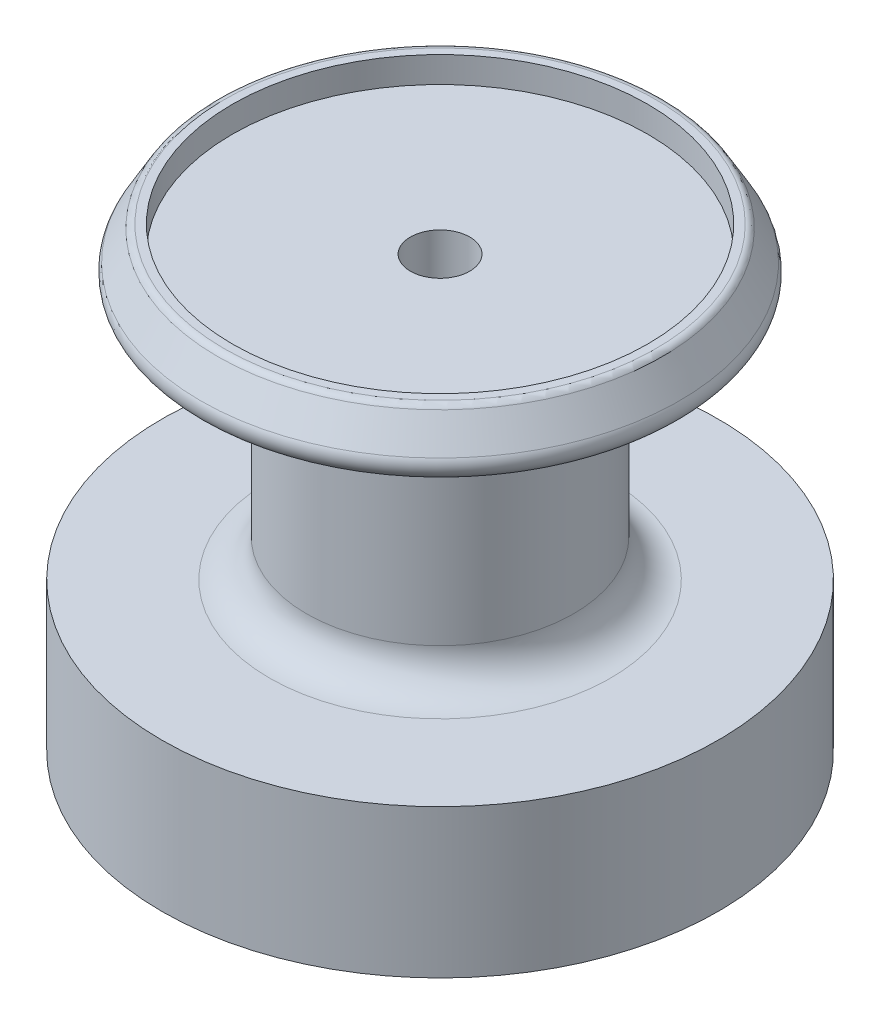
ISO-10303-21;
HEADER;
FILE_DESCRIPTION(('STEP AP214'),'2;1');
FILE_NAME('part.step','',(''),(''),'','','');
FILE_SCHEMA(('AUTOMOTIVE_DESIGN { 1 0 10303 214 1 1 1 1 }'));
ENDSEC;
DATA;
#1=APPLICATION_CONTEXT('core data for automotive mechanical design processes');
#2=APPLICATION_PROTOCOL_DEFINITION('international standard','automotive_design',2000,#1);
#3=PRODUCT_CONTEXT('',#1,'mechanical');
#4=PRODUCT('Part','Part','',(#3));
#5=PRODUCT_RELATED_PRODUCT_CATEGORY('part','',(#4));
#6=PRODUCT_DEFINITION_FORMATION('','',#4);
#7=PRODUCT_DEFINITION_CONTEXT('part definition',#1,'design');
#8=PRODUCT_DEFINITION('design','',#6,#7);
#9=PRODUCT_DEFINITION_SHAPE('','',#8);
#10=(LENGTH_UNIT() NAMED_UNIT(*) SI_UNIT(.MILLI.,.METRE.));
#11=(NAMED_UNIT(*) PLANE_ANGLE_UNIT() SI_UNIT($,.RADIAN.));
#12=(NAMED_UNIT(*) SI_UNIT($,.STERADIAN.) SOLID_ANGLE_UNIT());
#13=UNCERTAINTY_MEASURE_WITH_UNIT(LENGTH_MEASURE(1.E-05),#10,'distance_accuracy_value','');
#14=(GEOMETRIC_REPRESENTATION_CONTEXT(3) GLOBAL_UNCERTAINTY_ASSIGNED_CONTEXT((#13)) GLOBAL_UNIT_ASSIGNED_CONTEXT((#10,
#11,#12)) REPRESENTATION_CONTEXT('',''));
#15=CARTESIAN_POINT('',(0.,0.,0.));
#16=DIRECTION('',(0.,0.,1.));
#17=DIRECTION('',(1.,0.,0.));
#18=AXIS2_PLACEMENT_3D('',#15,#16,#17);
#19=CARTESIAN_POINT('',(0.,20.,0.));
#20=DIRECTION('',(0.,-1.,0.));
#21=DIRECTION('',(0.,0.,-1.));
#22=AXIS2_PLACEMENT_3D('',#19,#20,#21);
#23=CYLINDRICAL_SURFACE('',#22,37.5);
#24=CARTESIAN_POINT('',(0.,20.,0.));
#25=DIRECTION('',(0.,1.,0.));
#26=DIRECTION('',(0.,0.,1.));
#27=AXIS2_PLACEMENT_3D('',#24,#25,#26);
#28=CIRCLE('',#27,37.5);
#29=CARTESIAN_POINT('',(0.,20.,37.5));
#30=VERTEX_POINT('',#29);
#31=EDGE_CURVE('E62',#30,#30,#28,.T.);
#32=ORIENTED_EDGE('',*,*,#31,.F.);
#33=EDGE_LOOP('',(#32));
#34=FACE_BOUND('',#33,.T.);
#35=CARTESIAN_POINT('',(0.,0.,0.));
#36=DIRECTION('',(0.,1.,0.));
#37=DIRECTION('',(0.,0.,1.));
#38=AXIS2_PLACEMENT_3D('',#35,#36,#37);
#39=CIRCLE('',#38,37.5);
#40=CARTESIAN_POINT('',(0.,0.,37.5));
#41=VERTEX_POINT('',#40);
#42=EDGE_CURVE('E65',#41,#41,#39,.T.);
#43=ORIENTED_EDGE('',*,*,#42,.T.);
#44=EDGE_LOOP('',(#43));
#45=FACE_BOUND('',#44,.T.);
#46=ADVANCED_FACE('F40',(#34,#45),#23,.T.);
#47=CARTESIAN_POINT('',(0.,20.,0.));
#48=DIRECTION('',(0.,1.,0.));
#49=DIRECTION('',(0.,0.,1.));
#50=AXIS2_PLACEMENT_3D('',#47,#48,#49);
#51=PLANE('',#50);
#52=CARTESIAN_POINT('',(0.,20.,0.));
#53=DIRECTION('',(0.,1.,0.));
#54=DIRECTION('',(0.,0.,1.));
#55=AXIS2_PLACEMENT_3D('',#52,#53,#54);
#56=CIRCLE('',#55,23.);
#57=CARTESIAN_POINT('',(0.,20.,23.));
#58=VERTEX_POINT('',#57);
#59=EDGE_CURVE('E60',#58,#58,#56,.F.);
#60=ORIENTED_EDGE('',*,*,#59,.T.);
#61=EDGE_LOOP('',(#60));
#62=FACE_BOUND('',#61,.T.);
#63=ORIENTED_EDGE('',*,*,#31,.T.);
#64=EDGE_LOOP('',(#63));
#65=FACE_BOUND('',#64,.T.);
#66=ADVANCED_FACE('F148',(#62,#65),#51,.T.);
#67=CARTESIAN_POINT('',(0.,0.,0.));
#68=DIRECTION('',(0.,1.,0.));
#69=DIRECTION('',(0.,0.,1.));
#70=AXIS2_PLACEMENT_3D('',#67,#68,#69);
#71=PLANE('',#70);
#72=CARTESIAN_POINT('',(0.,0.,0.));
#73=DIRECTION('',(0.,-1.,0.));
#74=DIRECTION('',(0.,0.,-1.));
#75=AXIS2_PLACEMENT_3D('',#72,#73,#74);
#76=CIRCLE('',#75,35.);
#77=CARTESIAN_POINT('',(0.,0.,-35.));
#78=VERTEX_POINT('',#77);
#79=EDGE_CURVE('E79',#78,#78,#76,.T.);
#80=ORIENTED_EDGE('',*,*,#79,.F.);
#81=EDGE_LOOP('',(#80));
#82=FACE_BOUND('',#81,.T.);
#83=ORIENTED_EDGE('',*,*,#42,.F.);
#84=EDGE_LOOP('',(#83));
#85=FACE_BOUND('',#84,.T.);
#86=ADVANCED_FACE('F151',(#82,#85),#71,.F.);
#87=CARTESIAN_POINT('',(0.,54.,0.));
#88=DIRECTION('',(0.,-1.,0.));
#89=DIRECTION('',(0.,0.,-1.));
#90=AXIS2_PLACEMENT_3D('',#87,#88,#89);
#91=CYLINDRICAL_SURFACE('',#90,18.);
#92=CARTESIAN_POINT('',(0.,25.,0.));
#93=DIRECTION('',(0.,1.,0.));
#94=DIRECTION('',(0.,0.,1.));
#95=AXIS2_PLACEMENT_3D('',#92,#93,#94);
#96=CIRCLE('',#95,18.);
#97=CARTESIAN_POINT('',(0.,25.,18.));
#98=VERTEX_POINT('',#97);
#99=EDGE_CURVE('E58',#98,#98,#96,.T.);
#100=ORIENTED_EDGE('',*,*,#99,.T.);
#101=EDGE_LOOP('',(#100));
#102=FACE_BOUND('',#101,.T.);
#103=CARTESIAN_POINT('',(0.,54.,0.));
#104=DIRECTION('',(0.,1.,0.));
#105=DIRECTION('',(0.,0.,1.));
#106=AXIS2_PLACEMENT_3D('',#103,#104,#105);
#107=CIRCLE('',#106,18.);
#108=CARTESIAN_POINT('',(0.,54.,18.));
#109=VERTEX_POINT('',#108);
#110=EDGE_CURVE('E66',#109,#109,#107,.T.);
#111=ORIENTED_EDGE('',*,*,#110,.F.);
#112=EDGE_LOOP('',(#111));
#113=FACE_BOUND('',#112,.T.);
#114=ADVANCED_FACE('F158',(#102,#113),#91,.T.);
#115=CARTESIAN_POINT('',(0.,25.,0.));
#116=DIRECTION('',(0.,1.,0.));
#117=DIRECTION('',(0.,0.,1.));
#118=AXIS2_PLACEMENT_3D('',#115,#116,#117);
#119=TOROIDAL_SURFACE('',#118,23.,5.);
#120=ORIENTED_EDGE('',*,*,#59,.F.);
#121=EDGE_LOOP('',(#120));
#122=FACE_BOUND('',#121,.T.);
#123=ORIENTED_EDGE('',*,*,#99,.F.);
#124=EDGE_LOOP('',(#123));
#125=FACE_BOUND('',#124,.T.);
#126=ADVANCED_FACE('F141',(#122,#125),#119,.F.);
#127=CARTESIAN_POINT('',(0.,54.,0.));
#128=DIRECTION('',(0.,-1.,0.));
#129=DIRECTION('',(0.,0.,1.));
#130=AXIS2_PLACEMENT_3D('',#127,#128,#129);
#131=CONICAL_SURFACE('',#130,34.,0.523598775598299);
#132=CARTESIAN_POINT('',(0.,57.,0.));
#133=DIRECTION('',(0.,1.,0.));
#134=DIRECTION('',(0.,0.,1.));
#135=AXIS2_PLACEMENT_3D('',#132,#133,#134);
#136=CIRCLE('',#135,32.2679491924311);
#137=CARTESIAN_POINT('',(0.,57.,32.2679491924311));
#138=VERTEX_POINT('',#137);
#139=EDGE_CURVE('E42',#138,#138,#136,.T.);
#140=ORIENTED_EDGE('',*,*,#139,.T.);
#141=EDGE_LOOP('',(#140));
#142=FACE_BOUND('',#141,.T.);
#143=CARTESIAN_POINT('',(0.,61.,0.));
#144=DIRECTION('',(0.,-1.,0.));
#145=DIRECTION('',(0.,0.,-1.));
#146=AXIS2_PLACEMENT_3D('',#143,#144,#145);
#147=CIRCLE('',#146,29.9585481156726);
#148=CARTESIAN_POINT('',(0.,61.,-29.9585481156726));
#149=VERTEX_POINT('',#148);
#150=EDGE_CURVE('E48',#149,#149,#147,.T.);
#151=ORIENTED_EDGE('',*,*,#150,.T.);
#152=EDGE_LOOP('',(#151));
#153=FACE_BOUND('',#152,.T.);
#154=ADVANCED_FACE('F133',(#142,#153),#131,.T.);
#155=CARTESIAN_POINT('',(0.,61.5,0.));
#156=DIRECTION('',(0.,1.,0.));
#157=DIRECTION('',(0.,0.,1.));
#158=AXIS2_PLACEMENT_3D('',#155,#156,#157);
#159=PLANE('',#158);
#160=CARTESIAN_POINT('',(0.,61.5,0.));
#161=DIRECTION('',(0.,1.,0.));
#162=DIRECTION('',(0.,0.,1.));
#163=AXIS2_PLACEMENT_3D('',#160,#161,#162);
#164=CIRCLE('',#163,29.0925227118882);
#165=CARTESIAN_POINT('',(0.,61.5,29.0925227118882));
#166=VERTEX_POINT('',#165);
#167=EDGE_CURVE('E55',#166,#166,#164,.T.);
#168=ORIENTED_EDGE('',*,*,#167,.T.);
#169=EDGE_LOOP('',(#168));
#170=FACE_BOUND('',#169,.T.);
#171=CARTESIAN_POINT('',(0.,61.5,0.));
#172=DIRECTION('',(0.,1.,0.));
#173=DIRECTION('',(0.,0.,1.));
#174=AXIS2_PLACEMENT_3D('',#171,#172,#173);
#175=CIRCLE('',#174,28.);
#176=CARTESIAN_POINT('',(0.,61.5,28.));
#177=VERTEX_POINT('',#176);
#178=EDGE_CURVE('E74',#177,#177,#175,.T.);
#179=ORIENTED_EDGE('',*,*,#178,.F.);
#180=EDGE_LOOP('',(#179));
#181=FACE_BOUND('',#180,.T.);
#182=ADVANCED_FACE('F131',(#170,#181),#159,.T.);
#183=CARTESIAN_POINT('',(0.,54.,0.));
#184=DIRECTION('',(0.,1.,0.));
#185=DIRECTION('',(0.,0.,1.));
#186=AXIS2_PLACEMENT_3D('',#183,#184,#185);
#187=PLANE('',#186);
#188=CARTESIAN_POINT('',(0.,54.,0.));
#189=DIRECTION('',(0.,1.,0.));
#190=DIRECTION('',(0.,0.,1.));
#191=AXIS2_PLACEMENT_3D('',#188,#189,#190);
#192=CIRCLE('',#191,30.5358983848622);
#193=CARTESIAN_POINT('',(0.,54.,30.5358983848622));
#194=VERTEX_POINT('',#193);
#195=EDGE_CURVE('E10',#194,#194,#192,.F.);
#196=ORIENTED_EDGE('',*,*,#195,.T.);
#197=EDGE_LOOP('',(#196));
#198=FACE_BOUND('',#197,.T.);
#199=ORIENTED_EDGE('',*,*,#110,.T.);
#200=EDGE_LOOP('',(#199));
#201=FACE_BOUND('',#200,.T.);
#202=ADVANCED_FACE('F127',(#198,#201),#187,.F.);
#203=CARTESIAN_POINT('',(0.,58.,0.));
#204=DIRECTION('',(0.,1.,0.));
#205=DIRECTION('',(0.,0.,1.));
#206=AXIS2_PLACEMENT_3D('',#203,#204,#205);
#207=CYLINDRICAL_SURFACE('',#206,28.);
#208=CARTESIAN_POINT('',(0.,58.,0.));
#209=DIRECTION('',(0.,1.,0.));
#210=DIRECTION('',(0.,0.,1.));
#211=AXIS2_PLACEMENT_3D('',#208,#209,#210);
#212=CIRCLE('',#211,28.);
#213=CARTESIAN_POINT('',(0.,58.,28.));
#214=VERTEX_POINT('',#213);
#215=EDGE_CURVE('E75',#214,#214,#212,.T.);
#216=ORIENTED_EDGE('',*,*,#215,.F.);
#217=EDGE_LOOP('',(#216));
#218=FACE_BOUND('',#217,.T.);
#219=ORIENTED_EDGE('',*,*,#178,.T.);
#220=EDGE_LOOP('',(#219));
#221=FACE_BOUND('',#220,.T.);
#222=ADVANCED_FACE('F125',(#218,#221),#207,.F.);
#223=CARTESIAN_POINT('',(0.,58.,0.));
#224=DIRECTION('',(0.,1.,0.));
#225=DIRECTION('',(0.,0.,1.));
#226=AXIS2_PLACEMENT_3D('',#223,#224,#225);
#227=PLANE('',#226);
#228=CARTESIAN_POINT('',(0.,58.,0.));
#229=DIRECTION('',(0.,1.,0.));
#230=DIRECTION('',(0.,0.,1.));
#231=AXIS2_PLACEMENT_3D('',#228,#229,#230);
#232=CIRCLE('',#231,4.);
#233=CARTESIAN_POINT('',(0.,58.,4.));
#234=VERTEX_POINT('',#233);
#235=EDGE_CURVE('E101',#234,#234,#232,.T.);
#236=ORIENTED_EDGE('',*,*,#235,.F.);
#237=EDGE_LOOP('',(#236));
#238=FACE_BOUND('',#237,.T.);
#239=ORIENTED_EDGE('',*,*,#215,.T.);
#240=EDGE_LOOP('',(#239));
#241=FACE_BOUND('',#240,.T.);
#242=ADVANCED_FACE('F117',(#238,#241),#227,.T.);
#243=CARTESIAN_POINT('',(0.,60.5,0.));
#244=DIRECTION('',(0.,1.,0.));
#245=DIRECTION('',(0.,0.,1.));
#246=AXIS2_PLACEMENT_3D('',#243,#244,#245);
#247=TOROIDAL_SURFACE('',#246,29.0925227118882,1.);
#248=ORIENTED_EDGE('',*,*,#150,.F.);
#249=EDGE_LOOP('',(#248));
#250=FACE_BOUND('',#249,.T.);
#251=ORIENTED_EDGE('',*,*,#167,.F.);
#252=EDGE_LOOP('',(#251));
#253=FACE_BOUND('',#252,.T.);
#254=ADVANCED_FACE('F122',(#250,#253),#247,.T.);
#255=CARTESIAN_POINT('',(0.,56.,0.));
#256=DIRECTION('',(0.,1.,0.));
#257=DIRECTION('',(0.,0.,1.));
#258=AXIS2_PLACEMENT_3D('',#255,#256,#257);
#259=TOROIDAL_SURFACE('',#258,30.5358983848622,2.);
#260=ORIENTED_EDGE('',*,*,#195,.F.);
#261=EDGE_LOOP('',(#260));
#262=FACE_BOUND('',#261,.T.);
#263=ORIENTED_EDGE('',*,*,#139,.F.);
#264=EDGE_LOOP('',(#263));
#265=FACE_BOUND('',#264,.T.);
#266=ADVANCED_FACE('F39',(#262,#265),#259,.T.);
#267=CARTESIAN_POINT('',(0.,17.,0.));
#268=DIRECTION('',(0.,-1.,0.));
#269=DIRECTION('',(0.,0.,-1.));
#270=AXIS2_PLACEMENT_3D('',#267,#268,#269);
#271=CYLINDRICAL_SURFACE('',#270,35.);
#272=CARTESIAN_POINT('',(0.,17.,0.));
#273=DIRECTION('',(0.,-1.,0.));
#274=DIRECTION('',(0.,0.,-1.));
#275=AXIS2_PLACEMENT_3D('',#272,#273,#274);
#276=CIRCLE('',#275,35.);
#277=CARTESIAN_POINT('',(0.,17.,-35.));
#278=VERTEX_POINT('',#277);
#279=EDGE_CURVE('E77',#278,#278,#276,.T.);
#280=ORIENTED_EDGE('',*,*,#279,.F.);
#281=EDGE_LOOP('',(#280));
#282=FACE_BOUND('',#281,.T.);
#283=ORIENTED_EDGE('',*,*,#79,.T.);
#284=EDGE_LOOP('',(#283));
#285=FACE_BOUND('',#284,.T.);
#286=ADVANCED_FACE('F168',(#282,#285),#271,.F.);
#287=CARTESIAN_POINT('',(0.,17.,0.));
#288=DIRECTION('',(0.,-1.,0.));
#289=DIRECTION('',(0.,0.,-1.));
#290=AXIS2_PLACEMENT_3D('',#287,#288,#289);
#291=PLANE('',#290);
#292=CARTESIAN_POINT('',(0.,17.,0.));
#293=DIRECTION('',(0.,-1.,0.));
#294=DIRECTION('',(0.,0.,-1.));
#295=AXIS2_PLACEMENT_3D('',#292,#293,#294);
#296=CIRCLE('',#295,1.56211203184338);
#297=CARTESIAN_POINT('',(0.,17.,-1.56211203184338));
#298=VERTEX_POINT('',#297);
#299=EDGE_CURVE('E97',#298,#298,#296,.T.);
#300=ORIENTED_EDGE('',*,*,#299,.F.);
#301=EDGE_LOOP('',(#300));
#302=FACE_BOUND('',#301,.T.);
#303=CARTESIAN_POINT('',(0.,17.,-11.5));
#304=DIRECTION('',(0.,-1.,0.));
#305=DIRECTION('',(0.,0.,-1.));
#306=AXIS2_PLACEMENT_3D('',#303,#304,#305);
#307=CIRCLE('',#306,3.5);
#308=CARTESIAN_POINT('',(0.,17.,-15.));
#309=VERTEX_POINT('',#308);
#310=EDGE_CURVE('E95',#309,#309,#307,.T.);
#311=ORIENTED_EDGE('',*,*,#310,.F.);
#312=EDGE_LOOP('',(#311));
#313=FACE_BOUND('',#312,.T.);
#314=CARTESIAN_POINT('',(0.,17.,11.5));
#315=DIRECTION('',(0.,-1.,0.));
#316=DIRECTION('',(0.,0.,-1.));
#317=AXIS2_PLACEMENT_3D('',#314,#315,#316);
#318=CIRCLE('',#317,3.5);
#319=CARTESIAN_POINT('',(0.,17.,8.));
#320=VERTEX_POINT('',#319);
#321=EDGE_CURVE('E90',#320,#320,#318,.T.);
#322=ORIENTED_EDGE('',*,*,#321,.F.);
#323=EDGE_LOOP('',(#322));
#324=FACE_BOUND('',#323,.T.);
#325=ORIENTED_EDGE('',*,*,#279,.T.);
#326=EDGE_LOOP('',(#325));
#327=FACE_BOUND('',#326,.T.);
#328=ADVANCED_FACE('F176',(#302,#313,#324,#327),#291,.T.);
#329=CARTESIAN_POINT('',(0.,51.,11.5));
#330=DIRECTION('',(0.,-1.,0.));
#331=DIRECTION('',(0.,0.,-1.));
#332=AXIS2_PLACEMENT_3D('',#329,#330,#331);
#333=CYLINDRICAL_SURFACE('',#332,3.5);
#334=CARTESIAN_POINT('',(0.,51.,11.5));
#335=DIRECTION('',(0.,-1.,0.));
#336=DIRECTION('',(0.,0.,-1.));
#337=AXIS2_PLACEMENT_3D('',#334,#335,#336);
#338=CIRCLE('',#337,3.5);
#339=CARTESIAN_POINT('',(0.,51.,8.));
#340=VERTEX_POINT('',#339);
#341=EDGE_CURVE('E81',#340,#340,#338,.T.);
#342=ORIENTED_EDGE('',*,*,#341,.F.);
#343=EDGE_LOOP('',(#342));
#344=FACE_BOUND('',#343,.T.);
#345=ORIENTED_EDGE('',*,*,#321,.T.);
#346=EDGE_LOOP('',(#345));
#347=FACE_BOUND('',#346,.T.);
#348=ADVANCED_FACE('F183',(#344,#347),#333,.F.);
#349=CARTESIAN_POINT('',(0.,51.,11.5));
#350=DIRECTION('',(0.,-1.,0.));
#351=DIRECTION('',(0.,0.,-1.));
#352=AXIS2_PLACEMENT_3D('',#349,#350,#351);
#353=PLANE('',#352);
#354=ORIENTED_EDGE('',*,*,#341,.T.);
#355=EDGE_LOOP('',(#354));
#356=FACE_BOUND('',#355,.T.);
#357=ADVANCED_FACE('F188',(#356),#353,.T.);
#358=CARTESIAN_POINT('',(0.,51.,-11.5));
#359=DIRECTION('',(0.,-1.,0.));
#360=DIRECTION('',(0.,0.,-1.));
#361=AXIS2_PLACEMENT_3D('',#358,#359,#360);
#362=CYLINDRICAL_SURFACE('',#361,3.5);
#363=CARTESIAN_POINT('',(0.,51.,-11.5));
#364=DIRECTION('',(0.,-1.,0.));
#365=DIRECTION('',(0.,0.,-1.));
#366=AXIS2_PLACEMENT_3D('',#363,#364,#365);
#367=CIRCLE('',#366,3.5);
#368=CARTESIAN_POINT('',(0.,51.,-15.));
#369=VERTEX_POINT('',#368);
#370=EDGE_CURVE('E84',#369,#369,#367,.T.);
#371=ORIENTED_EDGE('',*,*,#370,.F.);
#372=EDGE_LOOP('',(#371));
#373=FACE_BOUND('',#372,.T.);
#374=ORIENTED_EDGE('',*,*,#310,.T.);
#375=EDGE_LOOP('',(#374));
#376=FACE_BOUND('',#375,.T.);
#377=ADVANCED_FACE('F192',(#373,#376),#362,.F.);
#378=CARTESIAN_POINT('',(0.,51.,0.));
#379=DIRECTION('',(0.,-1.,0.));
#380=DIRECTION('',(0.,0.,-1.));
#381=AXIS2_PLACEMENT_3D('',#378,#379,#380);
#382=PLANE('',#381);
#383=ORIENTED_EDGE('',*,*,#370,.T.);
#384=EDGE_LOOP('',(#383));
#385=FACE_BOUND('',#384,.T.);
#386=ADVANCED_FACE('F198',(#385),#382,.T.);
#387=CARTESIAN_POINT('',(0.,26.,0.));
#388=DIRECTION('',(0.,-1.,0.));
#389=DIRECTION('',(0.,0.,-1.));
#390=AXIS2_PLACEMENT_3D('',#387,#388,#389);
#391=CYLINDRICAL_SURFACE('',#390,1.56211203184338);
#392=CARTESIAN_POINT('',(0.,26.,0.));
#393=DIRECTION('',(0.,-1.,0.));
#394=DIRECTION('',(0.,0.,-1.));
#395=AXIS2_PLACEMENT_3D('',#392,#393,#394);
#396=CIRCLE('',#395,1.56211203184338);
#397=CARTESIAN_POINT('',(0.,26.,-1.56211203184338));
#398=VERTEX_POINT('',#397);
#399=EDGE_CURVE('E88',#398,#398,#396,.T.);
#400=ORIENTED_EDGE('',*,*,#399,.F.);
#401=EDGE_LOOP('',(#400));
#402=FACE_BOUND('',#401,.T.);
#403=ORIENTED_EDGE('',*,*,#299,.T.);
#404=EDGE_LOOP('',(#403));
#405=FACE_BOUND('',#404,.T.);
#406=ADVANCED_FACE('F204',(#402,#405),#391,.F.);
#407=CARTESIAN_POINT('',(0.,26.,0.));
#408=DIRECTION('',(0.,-1.,0.));
#409=DIRECTION('',(0.,0.,-1.));
#410=AXIS2_PLACEMENT_3D('',#407,#408,#409);
#411=PLANE('',#410);
#412=ORIENTED_EDGE('',*,*,#399,.T.);
#413=EDGE_LOOP('',(#412));
#414=FACE_BOUND('',#413,.T.);
#415=ADVANCED_FACE('F112',(#414),#411,.T.);
#416=CARTESIAN_POINT('',(0.,33.,0.));
#417=DIRECTION('',(0.,1.,0.));
#418=DIRECTION('',(0.,0.,1.));
#419=AXIS2_PLACEMENT_3D('',#416,#417,#418);
#420=CYLINDRICAL_SURFACE('',#419,4.);
#421=CARTESIAN_POINT('',(0.,33.,0.));
#422=DIRECTION('',(0.,1.,0.));
#423=DIRECTION('',(0.,0.,1.));
#424=AXIS2_PLACEMENT_3D('',#421,#422,#423);
#425=CIRCLE('',#424,4.);
#426=CARTESIAN_POINT('',(0.,33.,4.));
#427=VERTEX_POINT('',#426);
#428=EDGE_CURVE('E99',#427,#427,#425,.T.);
#429=ORIENTED_EDGE('',*,*,#428,.F.);
#430=EDGE_LOOP('',(#429));
#431=FACE_BOUND('',#430,.T.);
#432=ORIENTED_EDGE('',*,*,#235,.T.);
#433=EDGE_LOOP('',(#432));
#434=FACE_BOUND('',#433,.T.);
#435=ADVANCED_FACE('F111',(#431,#434),#420,.F.);
#436=CARTESIAN_POINT('',(0.,33.,0.));
#437=DIRECTION('',(0.,1.,0.));
#438=DIRECTION('',(0.,0.,1.));
#439=AXIS2_PLACEMENT_3D('',#436,#437,#438);
#440=PLANE('',#439);
#441=ORIENTED_EDGE('',*,*,#428,.T.);
#442=EDGE_LOOP('',(#441));
#443=FACE_BOUND('',#442,.T.);
#444=ADVANCED_FACE('F107',(#443),#440,.T.);
#445=CLOSED_SHELL('',(#46,#66,#86,#114,#126,#154,#182,#202,#222,#242,#254,#266,#286,#328,#348,
#357,#377,#386,#406,#415,#435,#444));
#446=MANIFOLD_SOLID_BREP('B2',#445);
#447=ADVANCED_BREP_SHAPE_REPRESENTATION('',(#18,#446),#14);
#448=SHAPE_DEFINITION_REPRESENTATION(#9,#447);
ENDSEC;
END-ISO-10303-21;
